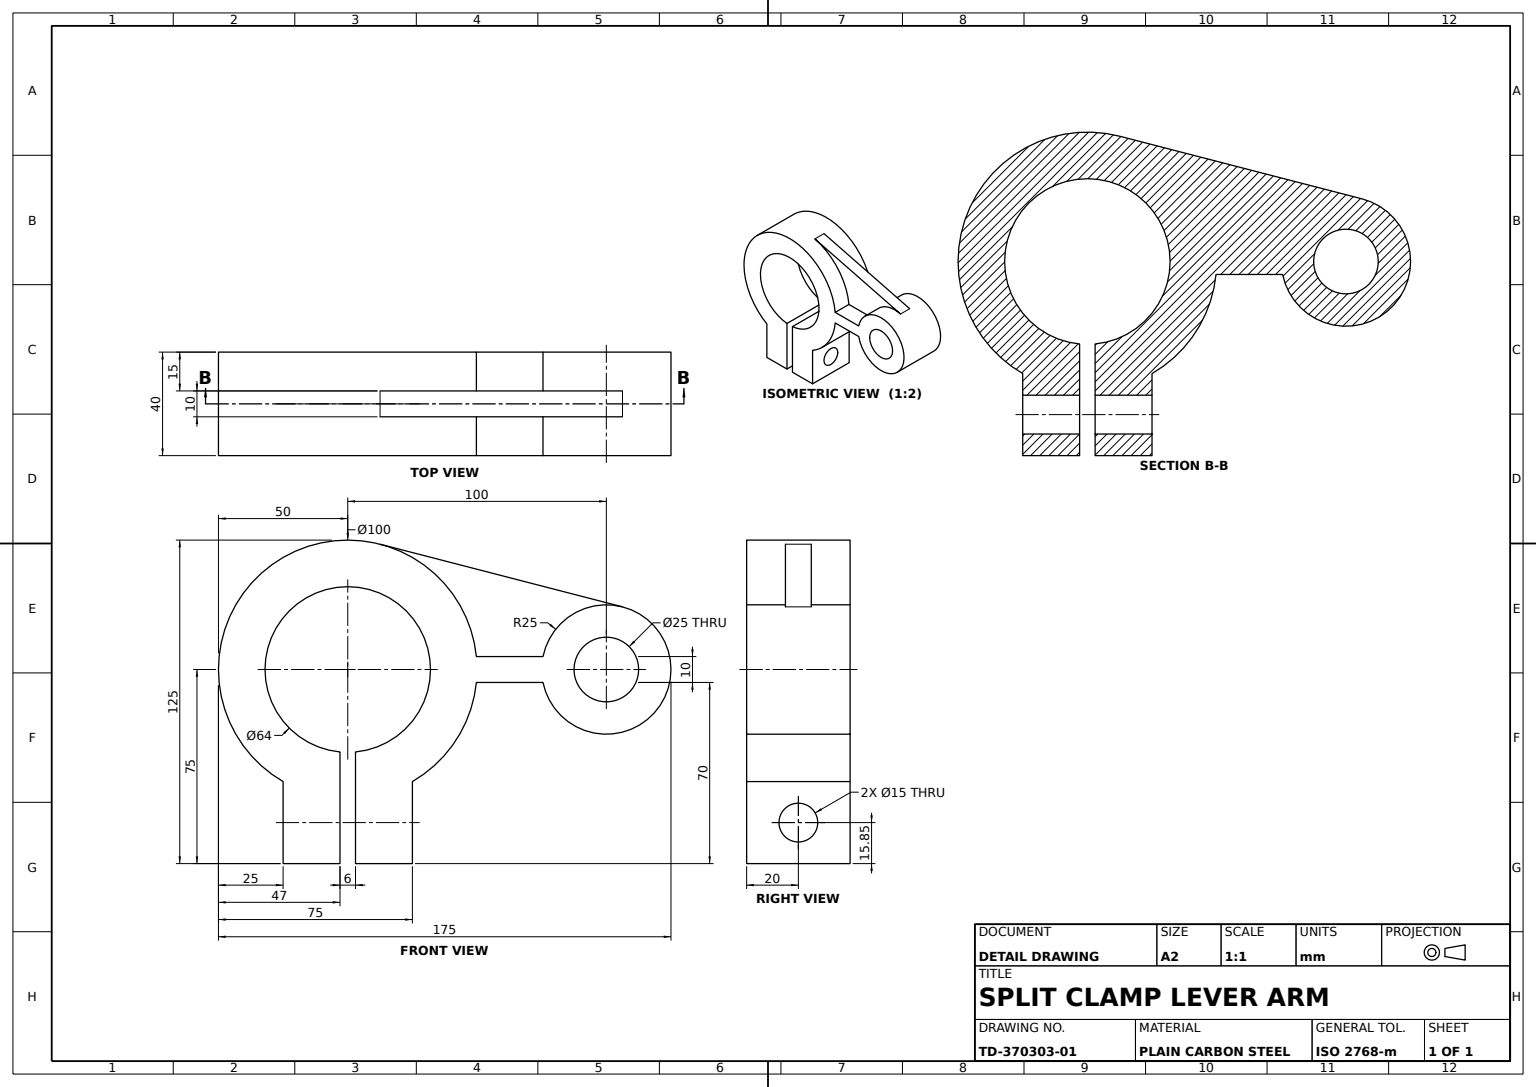
SolidWorks part; units mm, degrees
material "Plain Carbon Steel"
ref_plane "Front Plane" through (0, 0, 0) normal (0, 0, 1) x (1, 0, 0)
ref_plane "Top Plane" through (0, 0, 0) normal (0, 1, 0) x (1, 0, 0)
ref_plane "Right Plane" through (0, 0, 0) normal (1, 0, 0) x (0, 0, -1)
sketch "Clamp Ring Sketch" plane through (0, 0, 0) normal (0, 0, 1) x (1, 0, 0)
  circle A0 centre (0, 0) radius 32
  circle A1 centre (0, 0) radius 50
  dimension "D1" = 64
  dimension "D2" = 100
extrude "Clamp Ring Ø100 Bore Ø64" add sketch "Clamp Ring Sketch" along normal mid plane 40
sketch "Clamp Block and Secondary Boss Sketch" plane through (0, 0, 0) normal (0, 0, 1) x (1, 0, 0)
  line L1 (-25, -43.3013) -> (25, -43.3013)
  line L2 (-25, -43.3013) -> (-25, -75)
  line L3 (-25, -75) -> (25, -75)
  line L4 (25, -43.3013) -> (25, -75)
  circle A0 centre (100, 0) radius 25
  circle A1 centre (100, 0) radius 12.5
  circle A2 centre (0, 0) radius 50 construction
  point P10 (0, -75)
  dimension "D1" = 50
  dimension "D2" = 25
  dimension "D3" = 100
  dimension "D4" = 50
  dimension "D5" = 75
extrude "Clamp Block and Secondary Boss" add sketch "Clamp Block and Secondary Boss Sketch" along normal mid plane 40
sketch "Clamp Slot Sketch" plane through (0, 0, 0) normal (0, 0, 1) x (1, 0, 0)
  line L0 (-25, -75) -> (25, -75) construction
  line L1 (-3, -31.8591) -> (3, -31.8591)
  line L2 (-3, -31.8591) -> (-3, -75)
  line L3 (-3, -75) -> (3, -75)
  line L4 (3, -31.8591) -> (3, -75)
  circle A0 centre (0, 0) radius 32 construction
  point P8 (0, -75)
  dimension "D1" = 6
extrude "Clamp Slot 6mm" cut sketch "Clamp Slot Sketch" against normal through all both and the other way through all
sketch "Connecting Web Sketch" plane through (0, 0, 0) normal (0, 0, 1) x (1, 0, 0)
  line L0 (32, 0) -> (87.5, 0)
  circle A2 centre (100, 0) radius 12.5 construction
  arc A3 (3, -31.8591) -> (-3, -31.8591) centre (0, 0) ccw construction
extrude "Connecting Web 10mm" add sketch "Connecting Web Sketch" along normal mid plane 40 thin thin type mid plane wall 10
sketch "Stiffening Rib Sketch" plane through (0, 0, 0) normal (0, 0, 1) x (1, 0, 0)
  line L0 (106.25, 24.2061) -> (12.5, 48.4123)
  arc A1 (25, -43.3013) -> (49.7494, -5) centre (0, 0) ccw construction
  circle A2 centre (100, 0) radius 25 construction
rib "Stiffening Rib 10mm" sketch "Stiffening Rib Sketch" sketch "Stiffening Rib Sketch" thickness 10 extrusion direction parallel to sketch draft on no parameters "D1"=10
sketch "Clamp Bolt Hole Sketch" plane through (0, 0, 0) normal (1, 0, 0) x (0, 0, -1)
  line L2 (-20, -75) -> (-20, -43.3013) construction
  circle A0 centre (0, -59.1506) radius 7.5
  point P6 (-20, -59.1506)
  dimension "D1" = 15
extrude "Clamp Bolt Hole Ø15" cut sketch "Clamp Bolt Hole Sketch" against normal through all both and the other way through all
